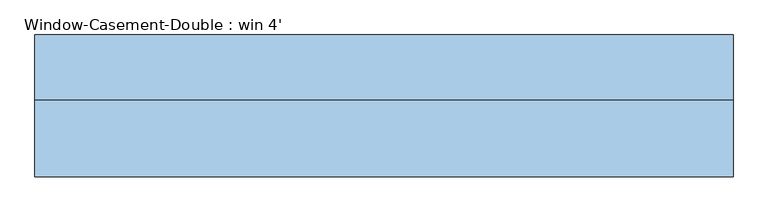
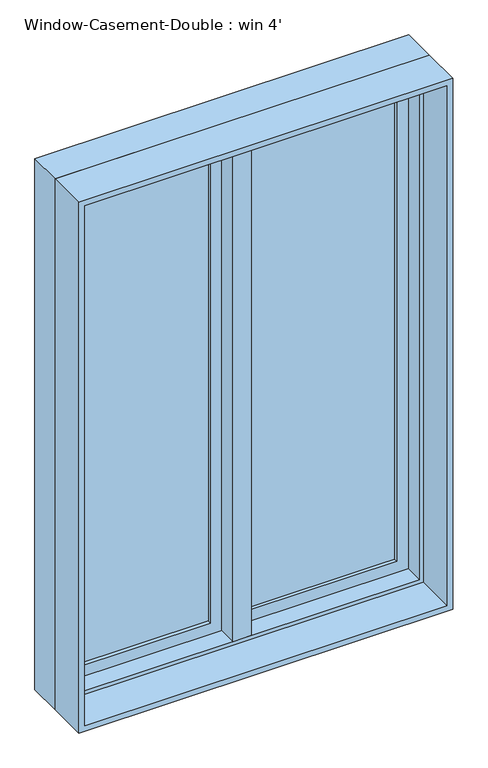
"""IFC4 building model written with IfcOpenShell, lengths in millimetres: window geometry, Window-Casement-Double : win 4'."""

from ifc_helpers import new_model, si_unit, frame, origin, place, context, project, spatial, polyline, outline, extrude, faceted_brep, source, transform, mapped, element, save


def window_casement_double_win_4_6ca1769e(model_context):
    return source(origin(), model_context, "Body", "SolidModel", [
        faceted_brep([(9.525, 133.35, 2730.5), (-9.525, 133.35, 2730.5), (-9.525, 82.55, 2730.5), (9.525, 82.55, 2730.5), (9.525, 133.35, 927.1), (9.525, 82.55, 927.1), (-9.525, 82.55, 927.1), (-9.525, 133.35, 927.1), (-9.525, 82.55, 946.15), (-9.525, 82.55, 2711.45), (-30.1625, 82.55, 946.15), (-30.1625, 82.55, 2711.45), (-30.1625, 19.05, 946.15), (-30.1625, 19.05, 2711.45), (30.1625, 19.05, 946.15), (30.1625, 19.05, 2711.45), (30.1625, 82.55, 946.15), (30.1625, 82.55, 2711.45), (9.525, 82.55, 946.15), (9.525, 82.55, 2711.45)], [[[0, 1, 2, 3]], [[4, 5, 6, 7]], [[1, 0, 4, 7]], [[2, 1, 7, 6, 8, 9]], [[9, 8, 10, 11]], [[11, 10, 12, 13]], [[13, 12, 14, 15]], [[15, 14, 16, 17]], [[17, 16, 18, 19]], [[0, 3, 19, 18, 5, 4]], [[18, 8, 6, 5]], [[9, 19, 3, 2]], [[8, 18, 16, 14, 12, 10]], [[19, 9, 11, 13, 15, 17]]]),
        extrude(outline(polyline([(-66.675, 114.3), (-66.675, 107.95), (-539.75, 107.95), (-539.75, 114.3), (-66.675, 114.3)])), frame((0.0, 0.0, 984.25), z_axis=(0.0, 0.0, 1.0), x_axis=(1.0, 0.0, 0.0)), (0.0, 0.0, 1.0), 1689.1),
        extrude(outline(polyline([(-539.75, 95.25), (-539.75, 101.6), (-66.675, 101.6), (-66.675, 95.25), (-539.75, 95.25)])), frame((0.0, 0.0, 984.25), z_axis=(0.0, 0.0, 1.0), x_axis=(1.0, 0.0, 0.0)), (0.0, 0.0, 1.0), 1689.1),
        extrude(outline(polyline([(539.75, 114.3), (539.75, 107.95), (66.675, 107.95), (66.675, 114.3), (539.75, 114.3)])), frame((0.0, 0.0, 984.25), z_axis=(0.0, 0.0, 1.0), x_axis=(1.0, 0.0, 0.0)), (0.0, 0.0, 1.0), 1689.1),
        extrude(outline(polyline([(66.675, 95.25), (66.675, 101.6), (539.75, 101.6), (539.75, 95.25), (66.675, 95.25)])), frame((0.0, 0.0, 984.25), z_axis=(0.0, 0.0, 1.0), x_axis=(1.0, 0.0, 0.0)), (0.0, 0.0, 1.0), 1689.1),
        extrude(outline(polyline([(2730.5, -596.9), (927.1, -596.9), (927.1, -9.525), (2730.5, -9.525), (2730.5, -596.9)]), holes=[polyline([(2673.35, -66.675), (984.25, -66.675), (984.25, -539.75), (2673.35, -539.75), (2673.35, -66.675)])]), frame((0.0, 82.55, 0.0), z_axis=(0.0, 1.0, 0.0), x_axis=(0.0, 0.0, 1.0)), (0.0, 0.0, 1.0), 44.45),
        extrude(outline(polyline([(927.1, 596.9), (2730.5, 596.9), (2730.5, 9.525), (927.1, 9.525), (927.1, 596.9)]), holes=[polyline([(984.25, 66.675), (2673.35, 66.675), (2673.35, 539.75), (984.25, 539.75), (984.25, 66.675)])]), frame((0.0, 82.55, 0.0), z_axis=(0.0, 1.0, 0.0), x_axis=(0.0, 0.0, 1.0)), (0.0, 0.0, 1.0), 44.45),
        extrude(outline(polyline([(2743.2, -609.6), (914.4, -609.6), (914.4, 609.6), (2743.2, 609.6), (2743.2, -609.6)]), holes=[polyline([(2724.15, 590.55), (933.45, 590.55), (933.45, -590.55), (2724.15, -590.55), (2724.15, 590.55)])]), frame((0.0, -114.3, 0.0), z_axis=(0.0, 1.0, 0.0), x_axis=(0.0, 0.0, 1.0)), (0.0, 0.0, 1.0), 133.35),
        faceted_brep([(577.85, 82.55, 2711.45), (577.85, 19.05, 2711.45), (-577.85, 19.05, 2711.45), (-577.85, 82.55, 2711.45), (596.9, 133.35, 2730.5), (596.9, 82.55, 2730.5), (-596.9, 82.55, 2730.5), (-596.9, 133.35, 2730.5), (609.6, 19.05, 2743.2), (609.6, 133.35, 2743.2), (-609.6, 133.35, 2743.2), (-609.6, 19.05, 2743.2), (-577.85, 19.05, 946.15), (-577.85, 82.55, 946.15), (-596.9, 82.55, 927.1), (-596.9, 133.35, 927.1), (-609.6, 133.35, 914.4), (-609.6, 19.05, 914.4), (577.85, 19.05, 946.15), (577.85, 82.55, 946.15), (596.9, 82.55, 927.1), (596.9, 133.35, 927.1), (609.6, 133.35, 914.4), (609.6, 19.05, 914.4)], [[[0, 1, 2, 3]], [[4, 5, 6, 7]], [[8, 9, 10, 11]], [[3, 2, 12, 13]], [[7, 6, 14, 15]], [[11, 10, 16, 17]], [[13, 12, 18, 19]], [[15, 14, 20, 21]], [[17, 16, 22, 23]], [[11, 17, 23, 8], [1, 18, 12, 2]], [[19, 18, 1, 0]], [[5, 20, 14, 6], [3, 13, 19, 0]], [[21, 20, 5, 4]], [[23, 22, 9, 8]], [[9, 22, 16, 10], [7, 15, 21, 4]]]),
    ])


if __name__ == "__main__":
    model = new_model("IFC4")
    model_context = context("Model", 3, world=origin())
    ifc_project = project(units=[si_unit("LENGTHUNIT", "METRE", prefix="MILLI")], contexts=[model_context])
    site = spatial("IfcSite", under=ifc_project)
    building = spatial("IfcBuilding", under=site)
    placement = place(None, origin())
    window_casement_double_win_4_shape = window_casement_double_win_4_6ca1769e(model_context)
    element("IfcWindow", 1, ObjectType="Window-Casement-Double : win 4'", at=placement, inside=building, context=model_context, shape_type="MappedRepresentation", body=[
        mapped(window_casement_double_win_4_shape, transform((0.0, 0.0, 0.0), x_axis=(1.0, 0.0, 0.0), y_axis=(0.0, 1.0, 0.0), z_axis=(0.0, 0.0, 1.0))),
    ])
    save(model, "model.ifc")

# Revit data of these elements
# Type "Window-Casement-Double : win 4'"
#   Type Mark = "19"
#   Fire Rating = "0.5h"
#   Assembly Code = "B2020100"
#   Analytic Construction = "Double glazing - domestic"
#   Frame Extension [instance default] = 0' - 0 1/4"
#   Window Inset [instance default] = 0' - 0"
#   Wall Thickness [instance default] = 0' - 6"
#   Interior Wall Closure [instance default] = 0' - 2 1/4"
#   Half Width = 2' - 0"
#   Visual Light Transmittance = 0.81
#   Thermal Resistance (R) = 1.8146 (h·ft²·°F)/BTU
#   Solar Heat Gain Coefficient = 0.76
#   Rough Width = 4' - 0 1/2"
#   Rough Height = 6' - 0 1/2"
#   Height = 6' - 0"
#   Heat Transfer Coefficient (U) = 0.5511 BTU/(h·ft²·°F)
#   Exterior Wall Closure [instance default] = 0' - 1 1/4"
#   Extension Jamb [instance default] = 0' - 2 1/4"
#   Default Sill Height = 3' - 0"
#   Width = 4' - 0"
#   Muntin Visibility = yes
#   Interior Trim Visibility [instance default] = yes
#   Exterior Trim Visibility [instance default] = yes
#   Extension Jamb Visibility [instance default] = yes
#   Interior Trim Material = Wood - Stained
#   Muntin Pattern = Muntin Pattern_2x2 : Muntin Pattern_2x2
#   Interior Trim = Trim-Window-Interior-Flat : Picture Frame
#   Interior Frame Material = Wood - Stained
#   Glass Panel Material = Glass
#   Exterior Trim Material = Clad - White
#   Exterior Trim = Trim-Window-Exterior-Flat : with Sill
#   Exterior Frame Material = Clad - White
#   Wall Closure = (empty or 0)
# Element 1 (IfcWindow, "Window-Casement-Double : win 4'")
#   Wall Thickness = 0' - 9"
#   Extension Jamb = 0' - 5 1/4"
#   Materials on its faces: "Wood - Stained", "Glass", "Clad - White"
# Materials
#   "Wood - Stained": class "Wood", colour RGB 224 178 126, transparency 0, Cost = 0
#   "Glass": class "Glass", colour RGB 0 128 192, transparency 0.75, Description = "Soda Lime Glass", Cost = 0
#   "Clad - White": class "Wood", colour RGB 242 242 238, transparency 0, Cost = 0
